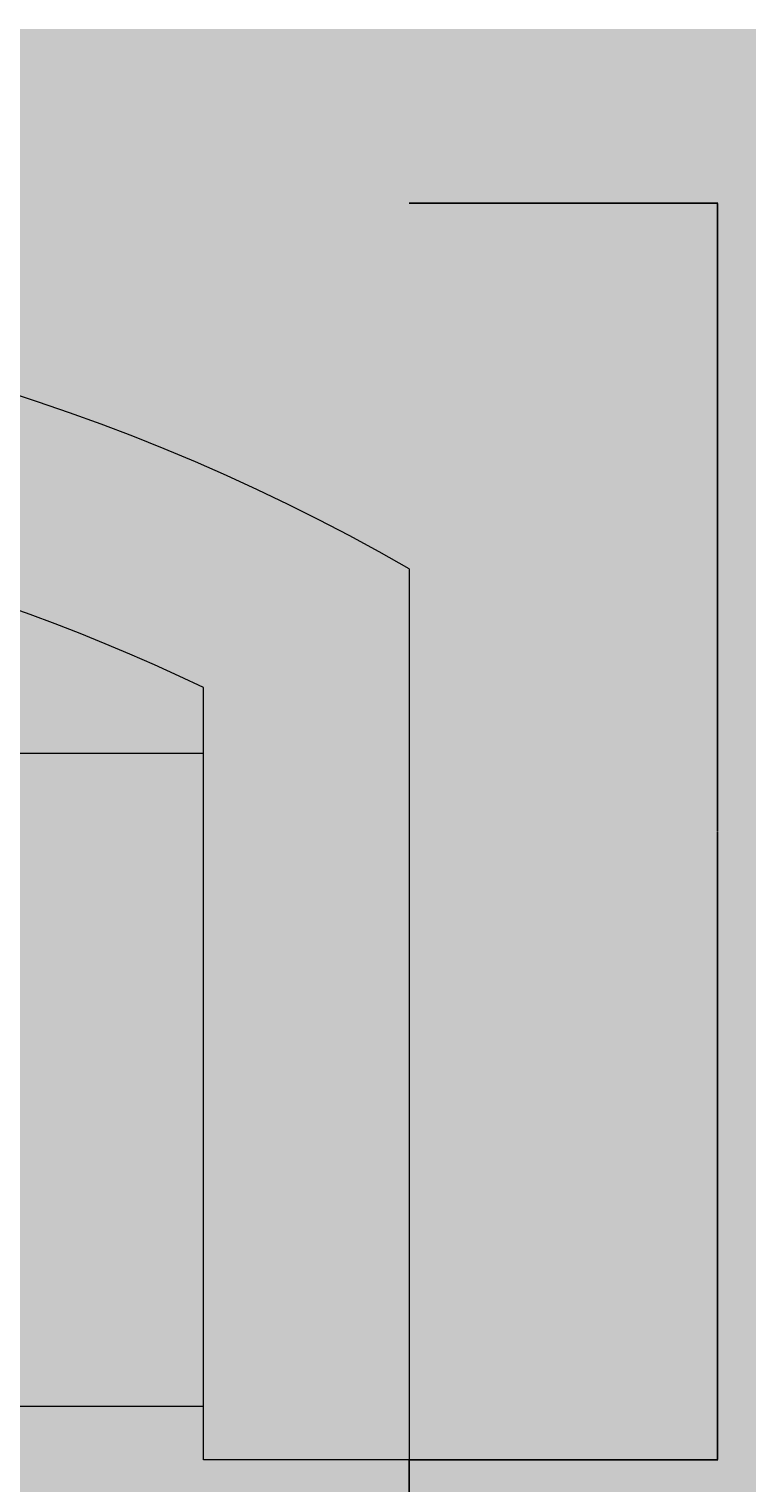
# Model space of a CAD drawing. Units: millimetres. Extents: x -229 to 16545, y -10488 to 4272.
# Tile 23 of 29: x 12629 to 13075, y -2111 to -1208. Entities that reach past the tile are written whole.
import ezdxf

# ---------------------------------------------------------------- set-up
doc = ezdxf.new("R2010")
doc.units = ezdxf.units.MM
for name, color, linetype, lineweight in [('A-ANNO-DIMS', 2, 'Continuous', 18), ('A-FURN', 8, 'Continuous', 18), ('A-FURN-PATT', 252, 'Continuous', 13)]:
    doc.layers.add(name, color=color, linetype=linetype, lineweight=lineweight)
doc.layers.add('A-FLOR-PATT', color=254, linetype='Continuous', lineweight=13, true_color=0xfeeab9)
doc.styles.get("Standard").update_dxf_attribs({"font": 'arial.ttf'})
doc.dimstyles.get("Standard").update_dxf_attribs({"dimtxt": 0.18, "dimasz": 0.18, "dimexe": 0.18, "dimexo": 0.0625, "dimgap": 0.09, "dimtad": 0, "dimtih": 1, "dimtoh": 1, "dimdec": 4, "dimzin": 0, "dimdsep": 46, "dimtxsty": 'Standard', "dimcen": 0.09, "dimadec": 0, "dimazin": 0, "dimtfac": 1, "dimtdec": 4, "dimtofl": 0, "dimtmove": 0, "dimatfit": 3, "dimfxl": 1, "dimtolj": 1, "dimtzin": 0, "dimarcsym": 0})

# ---------------------------------------------------------------- blocks, each defined once
blk = doc.blocks.new('Sofa - Roundback Loveseat 5 ft.')
for p, q in [((24.00004, -33.99998), (24.00004, -11.46958)), ((-23.9998, -13.38178), (23.99986, -13.38178)), ((-24, -32.44198), (24.00004, -32.44198))]:
    blk.add_line(p, q)
blk.add_lwpolyline([(30.00004, -7.99998), (30.00004, -33.99998), (24.00004, -33.99998)])
for centre, radius, start, end in [((0, -60.24998), 60.24998, 60.13715, 119.8628), ((0, -61.38438), 55.38444, 64.32083, 115.6792)]:
    blk.add_arc(centre, radius, start, end)
blk = doc.blocks.new('*D39')
at = {"layer": 'A-ANNO-DIMS', "color": 0, "lineweight": -2, "transparency": 16777216}
for p, q in [((11588.75, -2096.32), (11588.75, -2287.86)), ((12864.92, -2096.32), (12864.92, -2287.86)), ((11588.93, -2287.68), (12225.78, -2287.68)), ((12864.74, -2287.68), (12227.89, -2287.68))]:
    blk.add_line(p, q, dxfattribs=at)
at = {"layer": 'A-ANNO-DIMS', "color": 0, "transparency": 16777216}
for points in [[(11588.93, -2287.65), (11588.93, -2287.71), (11588.75, -2287.68)], [(12864.74, -2287.65), (12864.74, -2287.71), (12864.92, -2287.68)]]:
    blk.add_solid(points, dxfattribs=at)
at = {"layer": 'Defpoints', "color": 0, "transparency": 16777216}
for p in [(11588.75, -2096.26), (12864.92, -2096.26), (12864.92, -2287.68)]:
    blk.add_point(p, dxfattribs=at)
at = {"layer": 'A-ANNO-DIMS', "color": 0, "transparency": 16777216, "insert": (12226.83, -2287.68), "char_height": 0.18, "attachment_point": 5}
blk.add_mtext('\\A1;LOVESEAT 1276', dxfattribs=at)
blk = doc.blocks.new('*D40')
at = {"layer": 'A-ANNO-DIMS', "color": 0, "lineweight": -2, "transparency": 16777216}
for p, q in [((12864.98, -1316.38), (13056.52, -1316.38)), ((13056.34, -1316.56), (13056.34, -1706.14)), ((13056.34, -2096.08), (13056.34, -1706.5)), ((12864.98, -2096.26), (13056.52, -2096.26))]:
    blk.add_line(p, q, dxfattribs=at)
at = {"layer": 'A-ANNO-DIMS', "color": 0, "transparency": 16777216}
for points in [[(13056.31, -1316.56), (13056.37, -1316.56), (13056.34, -1316.38)], [(13056.31, -2096.08), (13056.37, -2096.08), (13056.34, -2096.26)]]:
    blk.add_solid(points, dxfattribs=at)
at = {"layer": 'Defpoints', "color": 0, "transparency": 16777216}
for p in [(12864.92, -1316.38), (13056.34, -1316.38), (12864.92, -2096.26)]:
    blk.add_point(p, dxfattribs=at)
at = {"layer": 'A-ANNO-DIMS', "color": 0, "transparency": 16777216, "insert": (13056.34, -1706.32), "char_height": 0.18, "attachment_point": 5}
blk.add_mtext('\\A1;780', dxfattribs=at)

msp = doc.modelspace()

# ---------------------------------------------------------------- hatches: boundary and pattern name
at = {"layer": 'A-FLOR-PATT', "transparency": 33554592}
h = msp.add_hatch(color=256, dxfattribs=at)
h.dxf.hatch_style = 1
h.paths.add_polyline_path([(7975.933, -5325.772), (7943.121, -5325.772), (7943.121, -4576.49, 0.4014527), (7225.933, -5325.772, 0.4014527), (6508.746, -4576.49), (6508.746, -5325.772), (6475.933, -5325.772), (6475.933, -5438.272), (5975.933, -5438.272), (5975.933, -7267.724), (5975.933, -7438.272), (6478.619, -7438.272), (6463.448, -7355.919), (6464.88, -7356.837), (6463.849, -7358.097), (6478.619, -7438.272), (6610.327, -7438.272), (6632.656, -7409.564), (6632.525, -7406.967), (6634.208, -7407.569), (6619.273, -7426.77), (6654.466, -7438.272), (7610.517, -7438.272), (7607.41, -7421.409), (7608.842, -7422.327), (7607.812, -7423.587), (7610.517, -7438.272), (7975.933, -7438.272)])
h.paths.add_polyline_path([(13785.933, -1208.272), (9555.933, -1208.272), (9555.933, -961.785), (9705.933, -961.785), (9705.933, -918.035), (10704.976, -918.035, 0.4014527), (9705.933, 38.215), (9555.933, 38.215), (9555.933, 2021.728), (5975.933, 2021.728), (5975.933, 755.492), (5745.933, 755.492), (5745.933, 1427.266), (2918.813, 1427.266), (2918.813, -492.942), (5013.319, -492.942), (5013.319, -978.272), (5745.933, -978.272), (5745.933, -397.513), (5975.933, -397.513), (5975.933, -1208.272), (4560.933, -1208.272), (4560.933, -1265.772), (4448.433, -1265.772), (4448.433, -1298.585), (4445.933, -1298.585), (3699.151, -1298.585, 0.4014527), (4448.433, -2015.772), (4560.933, -2015.772), (4560.933, -2384.177), (5745.933, -2384.177), (5799.402, -2384.177), (5799.402, -4518.272), (5975.933, -4518.272), (5975.933, -5208.272), (6475.933, -5208.272), (6475.933, -4575.772), (6508.746, -4575.772), (6508.746, -4576.49, -0.3564726), (7216.672, -5208.272), (7235.194, -5208.272, -0.3564726), (7943.121, -4576.49), (7943.121, -4575.772), (7975.933, -4575.772), (7975.933, -5208.272), (11176.247, -5208.272), (11159.44, -5191.465), (10520.768, -5191.465), (10520.768, -4888.936), (10571.19, -4888.936), (10571.19, -4872.129), (10772.876, -4872.129), (10772.876, -4888.936), (10789.683, -4888.936), (10789.683, -4872.129), (10991.368, -4872.129), (10991.368, -4888.936), (11041.79, -4888.936), (11041.79, -4872.129), (11058.597, -4872.129, -0.0909091), (11428.354, -4872.129), (11445.162, -4872.129), (11445.162, -4888.936), (11529.197, -4888.936), (11529.197, -5191.465), (11327.512, -5191.465), (11310.704, -5208.272), (13785.933, -5208.272)])
h.paths.add_polyline_path([(11047.216, -1630.944, -1), (11402.816, -1630.944, -1)], flags=16)
h.paths.add_polyline_path([(11148.816, -1630.944), (11225.016, -1554.744), (11301.216, -1630.944), (11225.016, -1707.144)], flags=0)
h.paths.add_polyline_path([(11199.616, -1630.944, -1), (11250.416, -1630.944, -1)], flags=0)
h.paths.add_polyline_path([(11588.751, -2096.259), (11588.751, -1543.254, -0.266667), (12864.918, -1543.254), (12864.918, -2096.259), (12737.302, -2096.259), (12737.302, -2063.121), (11716.368, -2063.121), (11716.368, -2096.259)], flags=16)
h.paths.add_polyline_path([(12012.696, -2489.42), (12600.997, -2489.42), (12600.997, -3666.022), (12012.696, -3666.022)], flags=16)
h.paths.add_polyline_path([(12176.41, -3599.403), (12174.938, -3609.076), (12173.789, -3618.819), (12173.09, -3628.559), (12172.973, -3638.221), (12173.89, -3652.852), (12175.008, -3657.025), (12172.909, -3643.473), (12173.142, -3624.297), (12175.386, -3605.273)], flags=0)
h.paths.add_polyline_path([(8026.289, -286.944), (7737.703, -287.19), (7734.87, -269.156), (8029.092, -268.905)], flags=16)
h.paths.add_polyline_path([(7733.453, -260.139), (7710.784, -115.865), (7557.191, -115.996), (7556.999, 109.744), (7412.687, 132.166), (7412.433, 429.206), (7556.707, 451.876), (7556.568, 614.769), (7412.256, 637.19), (7412.003, 934.231), (7556.276, 956.9), (7556.084, 1182.639), (7709.677, 1182.77), (7732.099, 1327.082), (8029.14, 1327.335), (8051.808, 1183.062), (8205.401, 1183.192), (8205.594, 957.454), (8349.906, 935.031), (8350.159, 637.99), (8205.885, 615.322), (8206.024, 452.43), (8350.336, 430.006), (8350.59, 132.965), (8206.316, 110.298), (8206.509, -115.442), (8052.916, -115.573), (8030.493, -259.885)], flags=16)
h.paths.add_polyline_path([(12261.416, -3475.554), (12262.632, -3486.776), (12264.032, -3497.007), (12265.554, -3506.365), (12267.136, -3514.968), (12268.719, -3522.935), (12271.304, -3535.59), (12273.606, -3548.078), (12275.271, -3561.064), (12275.93, -3574.938), (12275.325, -3590.3), (12273.425, -3607.964), (12270.795, -3625.658), (12268.066, -3641.063), (12266.318, -3649.679), (12265.456, -3653.626), (12263.984, -3659.846), (12264.032, -3659.566), (12264.342, -3658.241), (12264.807, -3656.37), (12265.456, -3653.626), (12266.318, -3649.679), (12267.409, -3644.302), (12268.668, -3637.664), (12270.019, -3630.037), (12271.384, -3621.695), (12272.69, -3612.908), (12273.857, -3603.948), (12274.81, -3595.088), (12275.47, -3586.601), (12275.782, -3578.689), (12275.757, -3571.292), (12275.423, -3564.275), (12274.816, -3557.512), (12273.964, -3550.872), (12272.896, -3544.224), (12271.645, -3537.439), (12270.24, -3530.385), (12267.543, -3517.181), (12264.612, -3501.247), (12261.849, -3481.059)], flags=0)
h.paths.add_polyline_path([(12332.136, -3408.03), (12333.483, -3416.79), (12335.077, -3424.54), (12336.915, -3431.355), (12338.991, -3437.32), (12341.266, -3442.55), (12343.694, -3447.166), (12346.229, -3451.292), (12348.826, -3455.051), (12351.438, -3458.563), (12357.476, -3466.491), (12363.61, -3476.575), (12368.309, -3489.762), (12369.929, -3503.427), (12369.842, -3516.511), (12368.43, -3530.867), (12365.816, -3545.835), (12362.382, -3559.786), (12360.968, -3564.487), (12363.063, -3557.021), (12364.898, -3549.566), (12366.473, -3542.077), (12367.773, -3534.631), (12368.781, -3527.301), (12369.483, -3520.162), (12369.863, -3513.291), (12369.906, -3506.759), (12369.599, -3500.643), (12368.93, -3494.999), (12367.924, -3489.796), (12366.61, -3484.994), (12365.024, -3480.542), (12363.19, -3476.399), (12361.141, -3472.516), (12358.909, -3468.847), (12356.525, -3465.347), (12354.02, -3461.954), (12351.438, -3458.563), (12345.462, -3450.529), (12339.923, -3439.996), (12335.85, -3428.296), (12332.68, -3412.888)], flags=0)
h.paths.add_polyline_path([(12385.287, -3334.612), (12384.977, -3342.409), (12385.02, -3349.196), (12385.4, -3355.066), (12386.104, -3360.105), (12387.112, -3364.41), (12388.412, -3368.071), (12389.987, -3371.181), (12391.823, -3373.832), (12393.919, -3376.097), (12396.337, -3377.978), (12399.153, -3379.462), (12402.445, -3380.531), (12406.289, -3381.172), (12410.758, -3381.371), (12415.935, -3381.106), (12421.893, -3380.368), (12428.658, -3379.159), (12436.069, -3377.55), (12443.907, -3375.635), (12451.961, -3373.505), (12460.015, -3371.254), (12467.853, -3368.971), (12475.263, -3366.749), (12482.029, -3364.68), (12491.877, -3361.657), (12497.701, -3360.107), (12501.639, -3359.288), (12510.135, -3358.326), (12519.662, -3365.412), (12524.243, -3378.911), (12523.764, -3390.7), (12520.746, -3401.577), (12514.248, -3415.634), (12511.518, -3420.418), (12515.856, -3412.154), (12519.153, -3405.024), (12521.516, -3398.804), (12523.049, -3393.276), (12523.865, -3388.212), (12524.059, -3383.441), (12523.7, -3378.958), (12522.853, -3374.815), (12521.576, -3371.054), (12519.931, -3367.722), (12517.982, -3364.865), (12515.786, -3362.529), (12513.405, -3360.758), (12510.877, -3359.588), (12508.136, -3358.982), (12505.086, -3358.897), (12501.639, -3359.288), (12497.701, -3360.107), (12493.183, -3361.309), (12487.988, -3362.851), (12476.403, -3366.408), (12463.335, -3370.326), (12447.372, -3374.788), (12431.759, -3378.604), (12418.504, -3380.974), (12405.811, -3381.624), (12394.725, -3378.025), (12388.039, -3368.367), (12385.583, -3357.877), (12384.826, -3346.204), (12385.428, -3331.059), (12385.953, -3325.719)], flags=0)
h.paths.add_polyline_path([(7880.016, 1173.969), (7880.373, 1175.495), (7880.433, 1175.851), (7879.484, 1171.818)], flags=0)
h.paths.add_polyline_path([(7802.33, 874.962), (7800.771, 885.032), (7798.932, 893.941), (7796.811, 901.774), (7794.419, 908.63), (7791.798, 914.639), (7789.002, 919.945), (7786.083, 924.686), (7783.093, 929.005), (7780.087, 933.043), (7774.996, 939.717), (7768.406, 949.37), (7762.174, 963.427), (7759.342, 978.002), (7758.629, 991.888), (7759.492, 1007.928), (7761.801, 1025.496), (7765.392, 1044.035), (7766.625, 1049.048), (7764.522, 1039.543), (7762.719, 1030.232), (7761.232, 1021.168), (7760.08, 1012.405), (7759.28, 1003.994), (7758.849, 995.988), (7758.806, 988.44), (7759.167, 981.404), (7759.942, 974.914), (7761.104, 968.936), (7762.617, 963.414), (7764.448, 958.299), (7766.559, 953.535), (7768.918, 949.073), (7771.487, 944.856), (7774.232, 940.835), (7777.115, 936.938), (7782.377, 930.041), (7787.845, 922.139), (7793.348, 911.698), (7798.042, 898.247), (7801.702, 880.527)], flags=0)
h.paths.add_polyline_path([(12519.068, -3228.534), (12519.615, -3236.235), (12520.529, -3242.343), (12521.78, -3247.103), (12523.337, -3250.758), (12525.171, -3253.556), (12527.248, -3255.709), (12529.522, -3257.296), (12531.95, -3258.361), (12534.486, -3258.949), (12537.082, -3259.11), (12539.694, -3258.888), (12542.277, -3258.329), (12544.781, -3257.478), (12547.173, -3256.388), (12549.46, -3255.129), (12550.455, -3254.517), (12555.825, -3251.109), (12557.835, -3249.942), (12565.181, -3246.404), (12574.565, -3253.032), (12576.931, -3265.022), (12576.627, -3277.425), (12575.416, -3290.819), (12574.851, -3295.392), (12575.708, -3287.593), (12576.322, -3280.806), (12576.688, -3274.939), (12576.812, -3269.899), (12576.688, -3265.593), (12576.322, -3261.932), (12575.708, -3258.822), (12574.851, -3256.172), (12573.753, -3253.905), (12572.439, -3252.005), (12570.943, -3250.474), (12569.293, -3249.309), (12567.523, -3248.513), (12565.658, -3248.083), (12563.732, -3248.022), (12561.777, -3248.328), (12559.814, -3248.989), (12557.835, -3249.942), (12555.825, -3251.109), (12553.77, -3252.413), (12551.652, -3253.78), (12549.46, -3255.129), (12543.167, -3258.594), (12532.661, -3259.485), (12524.685, -3253.923), (12520.949, -3245.152), (12519.138, -3233.042)], flags=0)
h.paths.add_polyline_path([(7741.293, 790.501), (7741.641, 799.467), (7741.584, 807.269), (7741.141, 814.015), (7740.329, 819.809), (7739.165, 824.757), (7737.667, 828.966), (7735.853, 832.541), (7733.74, 835.586), (7731.348, 838.188), (7728.71, 840.348), (7725.861, 842.052), (7722.836, 843.28), (7719.671, 844.015), (7716.4, 844.237), (7713.06, 843.932), (7709.684, 843.081), (7706.304, 841.686), (7702.923, 839.834), (7699.543, 837.629), (7696.164, 835.178), (7692.784, 832.585), (7684.718, 826.315), (7675.609, 820.63), (7664.001, 817.274), (7654.105, 821.884), (7647.171, 832.02), (7644.191, 846.522), (7646.321, 860.288), (7647.49, 864.223), (7645.946, 857.865), (7645.046, 852.044), (7644.827, 846.557), (7645.243, 841.404), (7646.221, 836.642), (7647.693, 832.318), (7649.587, 828.489), (7651.832, 825.206), (7654.359, 822.523), (7657.097, 820.49), (7659.984, 819.145), (7662.993, 818.452), (7666.108, 818.357), (7669.311, 818.809), (7672.583, 819.755), (7675.908, 821.139), (7679.268, 822.913), (7682.645, 825.021), (7686.025, 827.401), (7689.404, 829.958), (7692.784, 832.585), (7700.505, 838.509), (7709.871, 843.64), (7721.436, 844.698), (7733.277, 837.617), (7739.571, 825.214), (7741.557, 811.049), (7741.669, 795.575)], flags=0)
h.paths.add_polyline_path([(8377.641, 137.216), (8359.607, 134.382), (8359.356, 428.605), (8377.395, 425.802)], flags=16)
h.paths.add_polyline_path([(7650.715, 668.465), (7650.08, 677.319), (7649.023, 684.34), (7647.579, 689.811), (7645.785, 694.012), (7643.675, 697.228), (7641.286, 699.7), (7638.669, 701.521), (7635.876, 702.744), (7632.96, 703.419), (7629.974, 703.601), (7626.971, 703.344), (7624.004, 702.697), (7621.125, 701.717), (7618.375, 700.462), (7615.749, 699.013), (7614.561, 698.279), (7608.435, 694.382), (7606.125, 693.04), (7598.981, 689.594), (7589.669, 693.773), (7585.26, 702.856), (7584.221, 713.11), (7584.49, 724.584), (7585.863, 739.937), (7586.518, 745.277), (7585.539, 736.31), (7584.841, 728.507), (7584.424, 721.761), (7584.288, 715.966), (7584.433, 711.016), (7584.86, 706.807), (7585.567, 703.231), (7586.556, 700.186), (7587.821, 697.58), (7589.332, 695.397), (7591.053, 693.637), (7592.951, 692.3), (7594.989, 691.385), (7597.132, 690.895), (7599.346, 690.826), (7601.594, 691.18), (7603.851, 691.943), (7606.125, 693.04), (7608.435, 694.382), (7610.797, 695.885), (7613.229, 697.458), (7620.475, 701.929), (7632.001, 704.44), (7643.476, 699.417), (7648.536, 687.571), (7650.63, 673.661)], flags=0)
h.paths.add_polyline_path([(7385.628, 136.37), (7385.382, 424.956), (7403.416, 427.789), (7403.667, 133.567)], flags=16)
h.paths.add_polyline_path([(12993.884, -2257.186), (12959.588, -2257.186), (12959.588, -2125.099), (13531.966, -2125.099, -0.1904762), (13531.966, -3974.321), (12959.588, -3974.321), (12959.588, -3842.233), (12993.884, -3842.233)], flags=16)
h.paths.add_polyline_path([(13413.486, -3313.884), (13413.486, -2785.535), (13562.885, -2785.535, -0.0496282), (13562.885, -3313.884)], flags=0)
h.paths.add_polyline_path([(8377.21, 642.241), (8359.176, 639.407), (8358.925, 933.629), (8376.964, 930.826)], flags=16)
h.paths.add_polyline_path([(13086.058, -1864.83), (13086.058, -1449.84), (13501.048, -1449.84), (13501.048, -1864.83)], flags=16)
h.paths.add_polyline_path([(13305.814, -1862.197), (13302.103, -1859.624), (13298.088, -1857.068), (13293.799, -1854.536), (13289.262, -1852.031), (13284.504, -1849.559), (13279.554, -1847.125), (13274.439, -1844.735), (13269.17, -1842.389), (13263.701, -1840.081), (13257.97, -1837.797), (13251.914, -1835.525), (13245.472, -1833.252), (13238.582, -1830.968), (13231.18, -1828.66), (13223.206, -1826.315), (13209.182, -1822.458), (13204.584, -1821.48), (13217.962, -1824.773), (13235.072, -1829.804), (13248.777, -1834.349), (13260.829, -1838.869), (13274.479, -1844.63), (13289.675, -1852.101), (13302.553, -1859.704)], flags=0)
h.paths.add_polyline_path([(13428.104, -1820.994), (13419.007, -1818.141), (13409.95, -1815.4), (13400.766, -1812.747), (13391.271, -1810.151), (13376.087, -1806.251), (13370.618, -1805.019), (13386.304, -1808.794), (13405.087, -1813.928), (13423.014, -1819.354)], flags=0)
h.paths.add_polyline_path([(7385.197, 641.395), (7384.951, 929.98), (7402.986, 932.814), (7403.236, 638.592)], flags=16)
h.paths.add_polyline_path([(13262.537, -1725.526), (13253.246, -1724.74), (13244.516, -1724.117), (13235.94, -1723.625), (13223.267, -1723.062), (13217.598, -1722.912), (13231.966, -1723.397), (13248.733, -1724.359), (13266.899, -1725.895), (13272.802, -1726.502)], flags=0)
h.paths.add_polyline_path([(13191.893, -1641.137), (13208.675, -1640.506), (13214.057, -1640.258), (13197.763, -1640.936)], flags=0)
h.paths.add_polyline_path([(13097.524, -1608.457), (13114.284, -1609.031), (13120.126, -1609.105), (13103.045, -1608.71)], flags=0)
h.paths.add_polyline_path([(13465.328, -1521.577), (13473.906, -1517.015), (13481.761, -1511.636), (13492.562, -1502.076), (13495.327, -1497.933), (13485.818, -1508.858), (13470.208, -1519.547)], flags=0)
h.paths.add_polyline_path([(13175.015, -1500.891), (13184.046, -1501.807), (13192.721, -1502.52), (13201.114, -1503.034), (13209.273, -1503.351), (13217.244, -1503.476), (13225.078, -1503.41), (13232.821, -1503.16), (13240.524, -1502.728), (13248.233, -1502.117), (13255.993, -1501.322), (13263.825, -1500.293), (13271.746, -1498.974), (13279.775, -1497.305), (13287.928, -1495.229), (13296.222, -1492.688), (13304.675, -1489.622), (13313.304, -1485.975), (13322.089, -1481.727), (13330.859, -1477.028), (13339.408, -1472.063), (13347.526, -1467.02), (13355.006, -1462.087), (13364.86, -1455.202), (13367.224, -1453.299), (13358.544, -1459.754), (13343.348, -1469.775), (13326.143, -1479.767), (13309.023, -1488.045), (13292.249, -1494.129), (13276.009, -1498.264), (13260.299, -1500.88), (13244.401, -1502.51), (13228.945, -1503.378), (13213.316, -1503.508), (13197.047, -1502.876), (13180.088, -1501.481)], flags=0)
h.paths.add_polyline_path([(7733.501, 1336.101), (7736.303, 1354.14), (8024.889, 1354.386), (8027.723, 1336.352)], flags=16)
at = {"layer": 'A-FURN-PATT'}
h = msp.add_hatch(color=256, dxfattribs=at)
h.dxf.hatch_style = 1
h.paths.add_polyline_path([(13413.486, -2257.186), (12993.884, -2257.186), (12993.884, -2785.535), (13413.486, -2785.535)], flags=17)
h.paths.add_polyline_path([(13413.486, -2785.535), (12993.884, -2785.535), (12993.884, -3313.884), (13413.486, -3313.884)], flags=17)
h.paths.add_polyline_path([(13413.486, -3313.884), (12993.884, -3313.884), (12993.884, -3842.233), (13413.486, -3842.233)], flags=17)
h.paths.add_polyline_path([(13531.966, -2125.099), (12959.588, -2125.099), (12959.588, -2257.186), (13455.573, -2257.186, -0.1519478), (13455.573, -3842.233), (12959.588, -3842.233), (12959.588, -3974.321), (13531.966, -3974.321, 0.1904762)])
h.paths.add_polyline_path([(13455.573, -2257.186), (13413.486, -2257.186), (13413.486, -2785.535), (13562.885, -2785.535, 0.0506466)], flags=17)
h.paths.add_polyline_path([(13562.885, -2785.535), (13413.486, -2785.535), (13413.486, -3313.884), (13562.885, -3313.884, 0.0496282)], flags=17)
h.paths.add_polyline_path([(13562.885, -3313.884), (13413.486, -3313.884), (13413.486, -3842.233), (13455.573, -3842.233, 0.0506467)], flags=17)
h.paths.add_polyline_path([(11588.751, -1543.254), (11588.751, -2096.259), (11716.368, -2096.259), (11716.368, -1617.061, -0.2279232), (12737.302, -1617.061), (12737.302, -2096.259), (12864.918, -2096.259), (12864.918, -1543.254, 0.266667)])
h.paths.add_polyline_path([(12226.834, -1500.713, 0.1125187), (11716.368, -1617.061), (11716.368, -1657.721), (12226.834, -1657.721)], flags=17)
h.paths.add_polyline_path([(12737.302, -1617.061, 0.1125189), (12226.834, -1500.713), (12226.834, -1657.721), (12737.302, -1657.721)], flags=17)
h.paths.add_polyline_path([(12226.834, -1657.721), (11716.368, -1657.721), (11716.368, -2063.121), (12226.834, -2063.121)], flags=17)
h.paths.add_polyline_path([(12737.302, -1657.721), (12226.834, -1657.721), (12226.834, -2063.121), (12737.302, -2063.121)], flags=17)

# ---------------------------------------------------------------- block references
at = {"layer": 'A-FURN', "xscale": 21.26944187666239, "yscale": 21.26944187666239, "zscale": 21.26944187666239}
msp.add_blockref('Sofa - Roundback Loveseat 5 ft.', (12226.834, -1373.098), dxfattribs=at)

# ---------------------------------------------------------------- dimensions: what is measured, and where the dimension line sits
at = {"layer": 'A-ANNO-DIMS'}
dim = msp.add_linear_dim(base=(13056.343, -1316.379), p1=(12864.918, -2096.259), p2=(12864.918, -1316.379), angle=90, dimstyle='Standard', override={"dimdec": 0, "dimlfac": 1, "dimrnd": 0, "dimzin": 0, "dimdsep": 46, "dimlunit": 2}, dxfattribs=at)
dim.commit()
dim.dimension.update_dxf_attribs({"geometry": '*D40', "text_midpoint": (13056.343, -1706.319)})
dim = msp.add_linear_dim(base=(12864.918, -2287.684), p1=(11588.751, -2096.259), p2=(12864.918, -2096.259), text='LOVESEAT <>', dimstyle='Standard', override={"dimdec": 0, "dimlfac": 1, "dimrnd": 0, "dimzin": 0, "dimdsep": 46, "dimlunit": 2}, dxfattribs=at)
dim.commit()
dim.dimension.update_dxf_attribs({"geometry": '*D39', "text_midpoint": (12226.835, -2287.684)})

doc.saveas('drawing.dxf')
